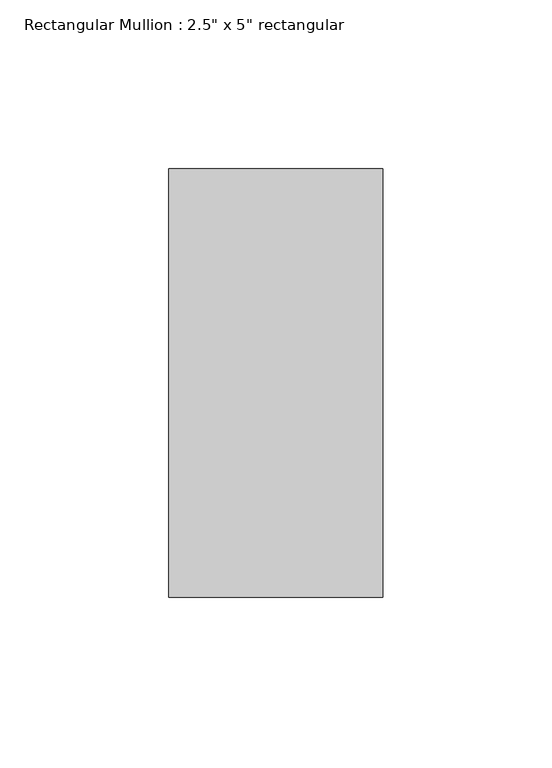
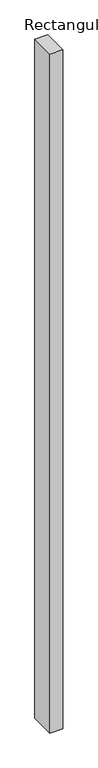
"""IFC4 building model written with IfcOpenShell, lengths in millimetres: member geometry."""

from ifc_helpers import new_model, si_unit, frame, origin, place, context, project, spatial, polyline, outline, extrude, source, transform, mapped, element, save


def member_58dfa4c6(model_context):
    return source(origin(), model_context, "Body", "SweptSolid", [
        extrude(outline(polyline([(31.75, 63.5), (31.75, -63.5), (-31.75, -63.5), (-31.75, 63.5), (31.75, 63.5)])), frame((0.0, 0.0, -3506.9820397), z_axis=(0.0, 0.0, 1.0), x_axis=(1.0, 0.0, 0.0)), (0.0, 0.0, 1.0), 3506.9820397),
    ])


if __name__ == "__main__":
    model = new_model("IFC4")
    model_context = context("Model", 3, world=origin())
    ifc_project = project(units=[si_unit("LENGTHUNIT", "METRE", prefix="MILLI")], contexts=[model_context])
    site = spatial("IfcSite", under=ifc_project)
    building = spatial("IfcBuilding", under=site)
    placement = place(None, origin())
    member_shape = member_58dfa4c6(model_context)
    element("IfcMember", 1, ObjectType="Rectangular Mullion : 2.5\" x 5\" rectangular", at=placement, inside=building, context=model_context, shape_type="MappedRepresentation", body=[
        mapped(member_shape, transform((0.0, 0.0, 0.0), x_axis=(1.0, 0.0, 0.0), y_axis=(0.0, 1.0, 0.0), z_axis=(0.0, 0.0, 1.0))),
    ])
    save(model, "model.ifc")

# Revit data of these elements
# Type "Rectangular Mullion : 2.5\" x 5\" rectangular"
#   built-in parameter 1007304 = 0.416667 (stored number, unit not read)
#   built-in parameter 1007301 = 0.104167 (stored number, unit not read)
#   built-in parameter 1007300 = 0.104167 (stored number, unit not read)
# Element 1 (IfcMember, "Rectangular Mullion : 2.5\" x 5\" rectangular")
#   Materials on its faces: "Damp-proofing"
# Materials
#   "Damp-proofing": class "Generic", colour RGB 127 127 127, transparency 0, Description = "Damp-proofing", Cost = 0
